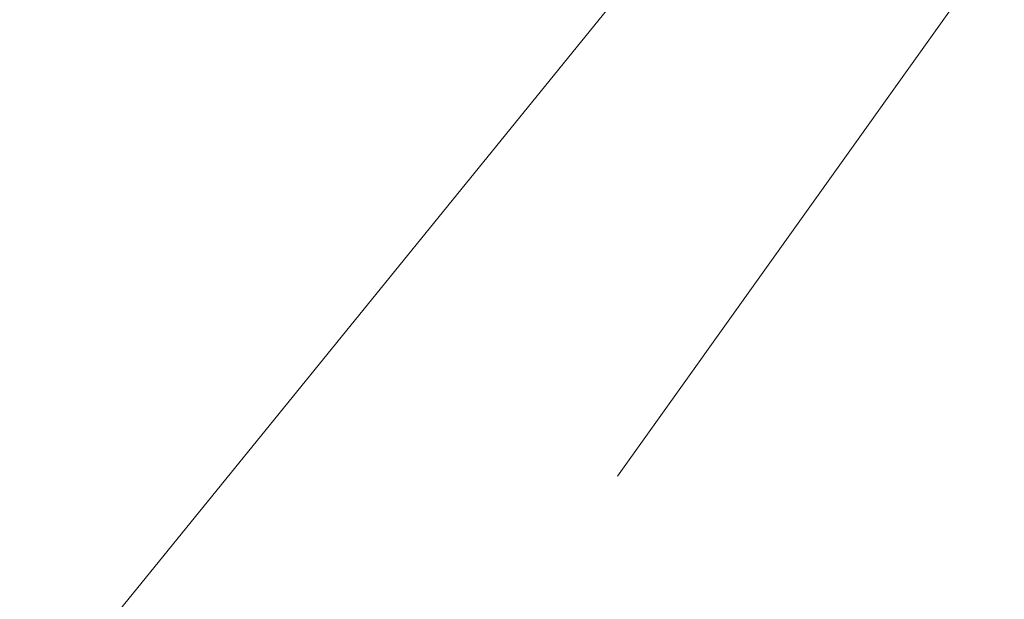
# Model space of a CAD drawing. Units: inches. Extents: x 375 to 1122, y 27 to 1069.
# Tile 94 of 155: x 728.243 to 731.282, y 861.878 to 863.668. Entities that reach past the tile are written whole.
import ezdxf

# ---------------------------------------------------------------- set-up
doc = ezdxf.new("R2010")
doc.units = ezdxf.units.IN
doc.layers.add('A-ANNO-DIMS', color=2, linetype='Continuous', lineweight=18)
doc.layers.add('Furniture', color=30, linetype='Continuous', lineweight=18)
doc.styles.get("Standard").update_dxf_attribs({"font": 'arial.ttf'})
doc.dimstyles.new('ISO-25', dxfattribs={"dimtxt": 12, "dimasz": 2.5, "dimexe": 1.5, "dimexo": 1.5, "dimtad": 1, "dimdec": 1, "dimlunit": 3, "dimtxsty": 'Standard', "dimblk": 'ARCHTICK', "dimcen": 2.5, "dimadec": 0, "dimazin": 0, "dimtfac": 1, "dimtdec": 1, "dimtmove": 0, "dimatfit": 3, "dimfxl": 1.5, "dimfxlon": 1, "dimarcsym": 0})

# ---------------------------------------------------------------- blocks, each defined once
blk = doc.blocks.new('A$C403C54AD')
for p, q in [((1.789224, 1.189932, 0.036628), (1.95298, 1.056939, 0.036628)), ((1.830163, 1.179702, 0.036628), (1.901807, 1.128551, 0.036628))]:
    blk.add_line(p, q)
blk = doc.blocks.new('_ArchTick')
at = {"color": 0, "linetype": 'ByBlock', "const_width": 0.15}
blk.add_lwpolyline([(-0.5, -0.5), (0.5, 0.5)], dxfattribs=at)
blk = doc.blocks.new('*D85')
at = {"layer": 'A-ANNO-DIMS', "color": 0, "lineweight": -2, "transparency": 16777216}
for p, q in [((401.5073, 868.5277), (398.5073, 868.5277)), ((400.0073, 814.5277), (400.0073, 868.5277)), ((401.5073, 814.5277), (398.5073, 814.5277))]:
    blk.add_line(p, q, dxfattribs=at)
at = {"layer": 'Defpoints', "color": 0, "transparency": 16777216}
for p in [(400.0073, 868.5277), (845.0073, 868.5277), (845.0073, 814.5277)]:
    blk.add_point(p, dxfattribs=at)
at = {"layer": 'A-ANNO-DIMS', "color": 0, "lineweight": -2, "transparency": 16777216, "xscale": 2.5, "yscale": 2.5, "zscale": 2.5}
for p, rotation in [((400.0073, 868.5277), 90), ((400.0073, 814.5277), 270)]:
    blk.add_blockref('_ArchTick', p, dxfattribs=dict(at, rotation=rotation))
at = {"layer": 'A-ANNO-DIMS', "color": 0, "transparency": 16777216, "insert": (393.2555, 841.5277), "char_height": 12, "attachment_point": 5, "rotation": 90}
blk.add_mtext('4\'-6"', dxfattribs=at)
blk = doc.blocks.new('*D88')
at = {"layer": 'A-ANNO-DIMS', "color": 0, "lineweight": -2, "transparency": 16777216}
for p, q in [((731.0073, 1052.5277), (731.0073, 1055.5277)), ((854.0073, 1052.5277), (854.0073, 1055.5277)), ((731.0073, 1054.0277), (854.0073, 1054.0277))]:
    blk.add_line(p, q, dxfattribs=at)
at = {"layer": 'Defpoints', "color": 0, "transparency": 16777216}
for p in [(854.0073, 1054.0277), (731.0073, 502.5277), (854.0073, 502.5277)]:
    blk.add_point(p, dxfattribs=at)
at = {"layer": 'A-ANNO-DIMS', "color": 0, "lineweight": -2, "transparency": 16777216, "xscale": 2.5, "yscale": 2.5, "zscale": 2.5, "rotation": 180}
blk.add_blockref('_ArchTick', (731.0073, 1054.0277), dxfattribs=at)
at = {"layer": 'A-ANNO-DIMS', "color": 0, "lineweight": -2, "transparency": 16777216, "xscale": 2.5, "yscale": 2.5, "zscale": 2.5}
blk.add_blockref('_ArchTick', (854.0073, 1054.0277), dxfattribs=at)
at = {"layer": 'A-ANNO-DIMS', "color": 0, "transparency": 16777216, "insert": (792.5073, 1060.7837), "char_height": 12, "attachment_point": 5}
blk.add_mtext('10\'-3"', dxfattribs=at)
blk = doc.blocks.new('*D91')
at = {"layer": 'A-ANNO-DIMS', "color": 0, "lineweight": -2, "transparency": 16777216}
for p, q in [((728.0073, 1052.5277), (728.0073, 1055.5277)), ((788.0073, 1052.5277), (788.0073, 1055.5277)), ((728.0073, 1054.0277), (788.0073, 1054.0277))]:
    blk.add_line(p, q, dxfattribs=at)
at = {"layer": 'Defpoints', "color": 0, "transparency": 16777216}
for p in [(788.0073, 1054.0277), (728.0073, 774.0277), (788.0073, 774.0277)]:
    blk.add_point(p, dxfattribs=at)
at = {"layer": 'A-ANNO-DIMS', "color": 0, "lineweight": -2, "transparency": 16777216, "xscale": 2.5, "yscale": 2.5, "zscale": 2.5, "rotation": 180}
blk.add_blockref('_ArchTick', (728.0073, 1054.0277), dxfattribs=at)
at = {"layer": 'A-ANNO-DIMS', "color": 0, "lineweight": -2, "transparency": 16777216, "xscale": 2.5, "yscale": 2.5, "zscale": 2.5}
blk.add_blockref('_ArchTick', (788.0073, 1054.0277), dxfattribs=at)
at = {"layer": 'A-ANNO-DIMS', "color": 0, "transparency": 16777216, "insert": (758.0073, 1060.7796), "char_height": 12, "attachment_point": 5}
blk.add_mtext('5\'-0"', dxfattribs=at)

msp = doc.modelspace()

# ---------------------------------------------------------------- block references
at = {"layer": 'Furniture', "xscale": 39.9918517141215, "yscale": 39.9918517141215, "zscale": 39.9918517141215, "rotation": 270}
msp.add_blockref('A$C403C54AD', (684.9549, 938.3156, 0.024), dxfattribs=at)

# ---------------------------------------------------------------- dimensions: what is measured, and where the dimension line sits
at = {"layer": 'A-ANNO-DIMS'}
for base, p1, p2, picture, middle in [((788.0073, 1054.0277), (728.0073, 774.0277), (788.0073, 774.0277), '*D91', (758.0073, 1060.7796)), ((854.0073, 1054.0277), (731.0073, 502.5277), (854.0073, 502.5277), '*D88', (792.5073, 1060.7837))]:
    dim = msp.add_linear_dim(base=base, p1=p1, p2=p2, dimstyle='ISO-25', override={"dimdec": 1, "dimlfac": 1, "dimrnd": 0, "dimzin": 1, "dimdsep": 46, "dimlunit": 4, "dimfrac": 2}, dxfattribs=at)
    dim.commit()
    dim.dimension.update_dxf_attribs({"geometry": picture, "text_midpoint": middle})
dim = msp.add_linear_dim(base=(400.0073, 868.5277), p1=(845.0073, 814.5277), p2=(845.0073, 868.5277), angle=90, dimstyle='ISO-25', override={"dimdec": 1, "dimlfac": 1, "dimrnd": 0, "dimzin": 1, "dimdsep": 46, "dimlunit": 4, "dimfrac": 2}, dxfattribs=at)
dim.commit()
dim.dimension.update_dxf_attribs({"geometry": '*D85', "text_midpoint": (393.2555, 841.5277)})

doc.saveas('drawing.dxf')
